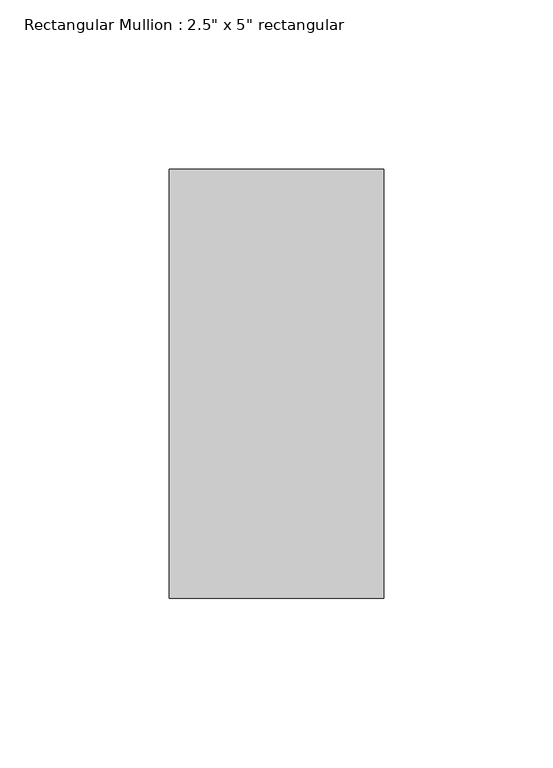
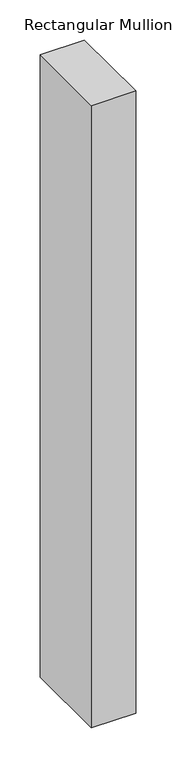
"""IFC4 building model written with IfcOpenShell, lengths in millimetres: member geometry."""

from ifc_helpers import new_model, si_unit, frame, origin, place, context, project, spatial, polyline, outline, extrude, source, transform, mapped, element, save


def member_6f38b482(model_context):
    return source(origin(), model_context, "Body", "SweptSolid", [
        extrude(outline(polyline([(0.0, 63.5), (0.0, -63.5), (-63.5, -63.5), (-63.5, 63.5), (0.0, 63.5)])), frame((0.0, 0.0, -944.4680153), z_axis=(0.0, 0.0, 1.0), x_axis=(1.0, 0.0, 0.0)), (0.0, 0.0, 1.0), 944.4680153),
    ])


if __name__ == "__main__":
    model = new_model("IFC4")
    model_context = context("Model", 3, world=origin())
    ifc_project = project(units=[si_unit("LENGTHUNIT", "METRE", prefix="MILLI")], contexts=[model_context])
    site = spatial("IfcSite", under=ifc_project)
    building = spatial("IfcBuilding", under=site)
    placement = place(None, origin())
    member_shape = member_6f38b482(model_context)
    element("IfcMember", 1, ObjectType="Rectangular Mullion : 2.5\" x 5\" rectangular", at=placement, inside=building, context=model_context, shape_type="MappedRepresentation", body=[
        mapped(member_shape, transform((0.0, 0.0, 0.0), x_axis=(1.0, 0.0, 0.0), y_axis=(0.0, 1.0, 0.0), z_axis=(0.0, 0.0, 1.0))),
    ])
    save(model, "model.ifc")

# Revit data of these elements
# Type "Rectangular Mullion : 2.5\" x 5\" rectangular"
#   built-in parameter 1007304 = 0.416667 (stored number, unit not read)
#   built-in parameter 1007301 = 0.104167 (stored number, unit not read)
#   built-in parameter 1007300 = 0.104167 (stored number, unit not read)
# Element 1 (IfcMember, "Rectangular Mullion : 2.5\" x 5\" rectangular")
#   Materials on its faces: "Aluminum"
# Materials
#   "Aluminum": class "Metal", colour RGB 247 247 247, transparency 0, Description = "Aluminum 6061", Cost = 0
